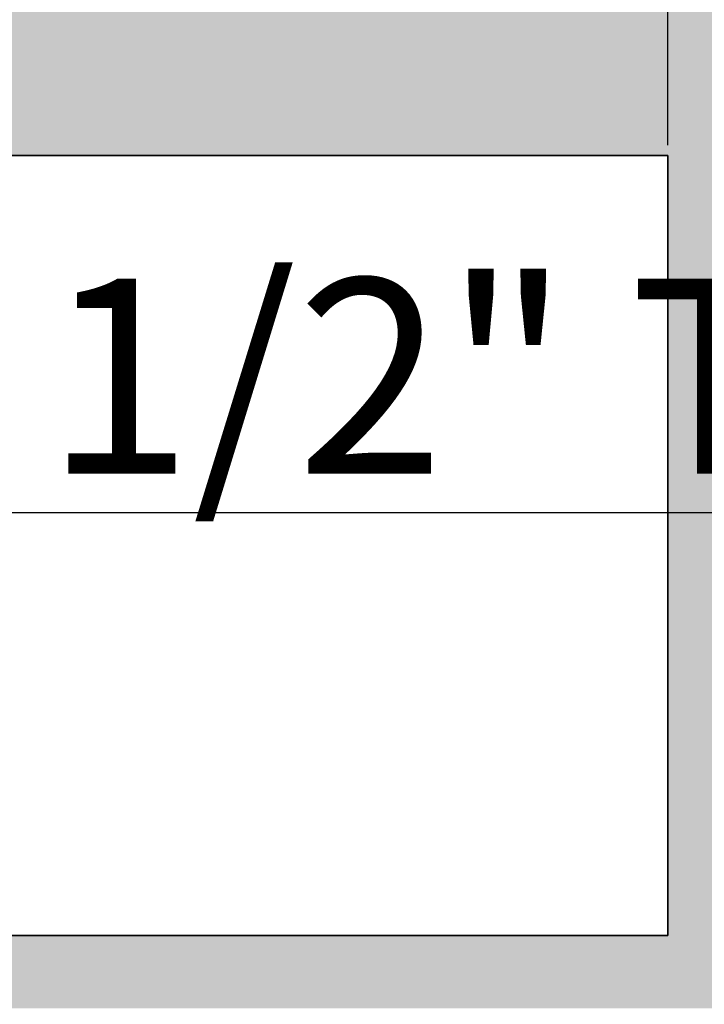
# Model space of a CAD drawing. Units: inches. Extents: x 2083 to 3317, y 1141 to 2115.
# Tile 20 of 256: x 2340 to 2382, y 1417 to 1477. Entities that reach past the tile are written whole.
import ezdxf

# ---------------------------------------------------------------- set-up
doc = ezdxf.new("R2010")
doc.units = ezdxf.units.IN
doc.layers.add('A-ANNO-DIMS', color=2, linetype='Continuous', lineweight=18)
doc.layers.add('A-WALL', color=7, linetype='Continuous', lineweight=35)
doc.layers.add('A-WALL-PATT', color=251, linetype='Continuous', lineweight=13, true_color=0x636466)
doc.styles.get("Standard").update_dxf_attribs({"font": 'arial.ttf'})
doc.dimstyles.new('ISO-25', dxfattribs={"dimtxt": 12, "dimasz": 12, "dimexe": 1.25, "dimexo": 0.625, "dimtad": 1, "dimlunit": 3, "dimtxsty": 'Standard', "dimcen": 2.5, "dimadec": 0, "dimazin": 0, "dimtfac": 1, "dimtmove": 0, "dimatfit": 3, "dimfxl": 1, "dimarcsym": 0})

# ---------------------------------------------------------------- blocks, each defined once
blk = doc.blocks.new('*D23')
at = {"layer": 'A-ANNO-DIMS', "color": 0, "lineweight": -2, "transparency": 16777216}
for p, q in [((2335.205, 1362.114), (2335.205, 1476.472)), ((2322.885, 1362.114), (2336.455, 1362.114)), ((2335.205, 1306.473), (2335.205, 1350.114)), ((2322.885, 1294.473), (2336.455, 1294.473))]:
    blk.add_line(p, q, dxfattribs=at)
at = {"layer": 'A-ANNO-DIMS', "color": 0, "transparency": 16777216}
for points in [[(2333.205, 1350.114), (2337.205, 1350.114), (2335.205, 1362.114)], [(2333.205, 1306.473), (2337.205, 1306.473), (2335.205, 1294.473)]]:
    blk.add_solid(points, dxfattribs=at)
at = {"layer": 'Defpoints', "color": 0, "transparency": 16777216}
for p in [(2322.26, 1362.114), (2335.205, 1362.114), (2322.26, 1294.473)]:
    blk.add_point(p, dxfattribs=at)
at = {"layer": 'A-ANNO-DIMS', "color": 0, "transparency": 16777216, "insert": (2328.376, 1425.293), "char_height": 12, "attachment_point": 5, "rotation": 90}
blk.add_mtext('5\'-7 1/2" TYP.', dxfattribs=at)
blk = doc.blocks.new('*D30')
at = {"layer": 'A-ANNO-DIMS', "color": 0, "lineweight": -2, "transparency": 16777216}
for p, q in [((2240.018, 1445.274), (2240.018, 1448.046)), ((2254.329, 1445.274), (2254.329, 1448.046)), ((2228.018, 1446.796), (2216.018, 1446.796)), ((2240.018, 1446.796), (2254.329, 1446.796)), ((2266.329, 1446.796), (2413.765, 1446.796))]:
    blk.add_line(p, q, dxfattribs=at)
at = {"layer": 'A-ANNO-DIMS', "color": 0, "transparency": 16777216}
for points in [[(2228.018, 1448.796), (2228.018, 1444.796), (2240.018, 1446.796)], [(2266.329, 1448.796), (2266.329, 1444.796), (2254.329, 1446.796)]]:
    blk.add_solid(points, dxfattribs=at)
at = {"layer": 'Defpoints', "color": 0, "transparency": 16777216}
for p in [(2254.329, 1446.796), (2240.018, 1444.649), (2254.329, 1444.649)]:
    blk.add_point(p, dxfattribs=at)
at = {"layer": 'A-ANNO-DIMS', "color": 0, "transparency": 16777216, "insert": (2346.047, 1453.625), "char_height": 12, "attachment_point": 5}
blk.add_mtext('WC 1\'-2 1/2" TYP.', dxfattribs=at)
blk = doc.blocks.new('*D62')
at = {"layer": 'A-ANNO-DIMS', "color": 0, "lineweight": -2, "transparency": 16777216}
for p, q in [((2235.96, 1469.386), (2235.96, 1522.361)), ((2379.96, 1469.386), (2379.96, 1522.361)), ((2247.96, 1521.111), (2367.96, 1521.111))]:
    blk.add_line(p, q, dxfattribs=at)
at = {"layer": 'A-ANNO-DIMS', "color": 0, "transparency": 16777216}
for points in [[(2247.96, 1523.111), (2247.96, 1519.111), (2235.96, 1521.111)], [(2367.96, 1523.111), (2367.96, 1519.111), (2379.96, 1521.111)]]:
    blk.add_solid(points, dxfattribs=at)
at = {"layer": 'Defpoints', "color": 0, "transparency": 16777216}
for p in [(2379.96, 1521.111), (2235.96, 1468.761), (2379.96, 1468.761)]:
    blk.add_point(p, dxfattribs=at)
at = {"layer": 'A-ANNO-DIMS', "color": 0, "transparency": 16777216, "insert": (2307.96, 1527.863), "char_height": 12, "attachment_point": 5}
blk.add_mtext('12\'-0"', dxfattribs=at)

msp = doc.modelspace()

# ---------------------------------------------------------------- hatches: boundary and pattern name
at = {"layer": 'A-WALL-PATT'}
h = msp.add_hatch(color=256, dxfattribs=at)
h.dxf.hatch_style = 1
h.paths.add_polyline_path([(3126.96, 2020.761), (2748.96, 2020.761), (2604.96, 2020.761), (2226.96, 2020.761), (2226.96, 1702.761), (2466.96, 1702.761), (2466.96, 1582.761), (2418.96, 1582.761), (2418.96, 1477.761), (2226.96, 1477.761), (2226.96, 1263.261), (2544.96, 1263.261), (2544.96, 1411.761), (2604.96, 1411.761), (2685.96, 1411.761), (2685.96, 1420.761), (2604.96, 1420.761), (2604.96, 1573.761), (2604.96, 1702.761), (2604.96, 2011.761), (2748.96, 2011.761), (2748.96, 1702.761), (2862.96, 1702.761), (2862.96, 1621.761), (2871.96, 1621.761), (2871.96, 1702.761), (2883.96, 1702.761), (2883.96, 1706.939, -0.026459), (2883.96, 1711.761), (2757.96, 1711.761), (2757.96, 1807.761), (2787.96, 1807.761), (2787.96, 1812.261), (2757.96, 1812.261), (2757.96, 2011.761), (2877.96, 2011.761), (2877.96, 1812.261), (2847.96, 1812.261), (2847.96, 1807.761), (2889.836, 1807.761), (2889.836, 1812.261), (2882.46, 1812.261), (2882.46, 2011.761), (3117.96, 2011.761), (3117.96, 1812.261), (2937.836, 1812.261), (2937.836, 1807.761), (2995.71, 1807.761), (2995.71, 1796.118), (3000.21, 1796.118), (3000.21, 1807.761), (3117.96, 1807.761), (3117.96, 1711.761), (3000.21, 1711.761), (3000.21, 1760.118), (2998.573, 1760.118, -0.020711), (2995.71, 1760.118), (2995.71, 1711.761), (2931.96, 1711.761), (2931.96, 1702.761), (3126.96, 1702.761)])
h.paths.add_polyline_path([(2471.46, 2011.761), (2471.46, 1810.011), (2462.717, 1810.011), (2462.717, 1805.511), (2505.96, 1805.511), (2505.96, 1810.011), (2475.96, 1810.011), (2475.96, 2011.761), (2595.96, 2011.761), (2595.96, 1810.011), (2565.96, 1810.011), (2565.96, 1805.511), (2595.96, 1805.511), (2595.96, 1711.761), (2235.96, 1711.761), (2235.96, 1805.511), (2353.71, 1805.511), (2353.71, 1796.054), (2358.21, 1796.054), (2358.21, 1805.511), (2414.717, 1805.511), (2414.717, 1810.011), (2235.96, 1810.011), (2235.96, 2011.761)], flags=16)
h.paths.add_polyline_path([(2270.205, 1994.61), (2270.205, 1970.61), (2246.205, 1970.61), (2246.205, 1994.61)], flags=0)
edge = h.paths.add_edge_path(flags=0)
edge.add_ellipse((2332.027, 1899.798), major_axis=(-3.043, 3.043), ratio=0.168252, start_angle=-161.33217, end_angle=-156.30711, ccw=False)
edge.add_ellipse((2333.082, 1898.744), major_axis=(-1.055, 1.055), ratio=0.453532, start_angle=-123.37102, end_angle=-94.15911)
edge = h.paths.add_edge_path(flags=0)
edge.add_ellipse((2332.027, 1968.876), major_axis=(3.043, 3.043), ratio=0.168252, start_angle=18.66783, end_angle=23.69289)
edge.add_spline(control_points=[(2332.926, 1970.691), (2332.227, 1970.336), (2330.894, 1969.659), (2328.413, 1970.932), (2327.204, 1967.749), (2324.71, 1969.956), (2322.533, 1967.012), (2320.013, 1971.296), (2317.68, 1968.158), (2316.041, 1967.102), (2315.427, 1966.81)], knot_values=[0, 0, 0, 0, 2.267059, 4.324559, 6.685584, 8.878641, 11.121502, 14.300359, 17.755284, 19.732645, 19.732645, 19.732645, 19.732645], degree=3, periodic=0)
edge.add_ellipse((2332.027, 1968.876), major_axis=(3.043, 3.043), ratio=0.168252, start_angle=18.66783, end_angle=23.69289, ccw=False)
edge.add_ellipse((2333.082, 1969.931), major_axis=(1.055, 1.055), ratio=0.453532, start_angle=56.62898, end_angle=85.84089, ccw=False)
edge = h.paths.add_edge_path(flags=0)
edge.add_spline(control_points=[(2296.428, 1967.988), (2293.628, 1965.336), (2287.704, 1959.727), (2299.744, 1949.996), (2294.533, 1935.669), (2290.573, 1920.604), (2293.394, 1909.974), (2296.185, 1904.967)], knot_values=[0.099185, 0.099185, 0.099185, 0.099185, 0.345301, 0.619822, 0.982653, 1.386093, 1.810555, 1.810555, 1.810555, 1.810555], degree=3, periodic=0)
edge.add_spline(control_points=[(2296.185, 1904.967), (2297.384, 1902.619), (2298.001, 1901.949), (2298.553, 1901.468)], knot_values=[0.006246, 0.006246, 0.006246, 0.006246, 0.055476, 0.055476, 0.055476, 0.055476], degree=3, periodic=0)
edge.add_spline(control_points=[(2298.553, 1901.468), (2297.259, 1900.923), (2295.225, 1900.232), (2293.06, 1900.614), (2292.101, 1900.788), (2292.09, 1900.791)], knot_values=[0.312835, 0.312835, 0.312835, 0.312835, 0.40178, 0.474987, 0.475903, 0.475903, 0.475903, 0.475903], degree=3, periodic=0)
edge.add_arc((2292.794, 1904.664), 3.937, 215.4209, 259.69818, ccw=False)
edge.add_spline(control_points=[(2289.585, 1902.382), (2289.477, 1902.535), (2289.368, 1902.688), (2289.261, 1902.841)], knot_values=[0.102872, 0.102872, 0.102872, 0.102872, 0.116896, 0.116896, 0.116896, 0.116896], degree=3, periodic=0)
edge.add_spline(control_points=[(2289.261, 1902.841), (2288.687, 1902.55), (2287.64, 1902.02), (2285.881, 1901.874), (2283.853, 1901.504), (2281.72, 1899.711), (2278.467, 1899.493), (2276.157, 1901.883), (2272.259, 1899.804), (2267.778, 1901.843), (2262.244, 1900.184), (2257.415, 1901.782), (2254.318, 1900.726), (2253.178, 1900.337)], knot_values=[0, 0, 0, 0, 1.907977, 3.477176, 5.261074, 7.972851, 11.680248, 13.717921, 16.939592, 22.789562, 27.502503, 33.595215, 37.145618, 37.145618, 37.145618, 37.145618], degree=3, periodic=0)
edge.add_line((2253.178, 1900.337), (2250.244, 1902.841))
edge.add_line((2250.244, 1902.841), (2250.244, 1965.833))
edge.add_line((2250.244, 1965.833), (2253.178, 1968.337))
edge.add_spline(control_points=[(2253.178, 1968.337), (2254.318, 1967.948), (2257.415, 1966.892), (2262.244, 1968.49), (2267.778, 1966.831), (2271.527, 1968.537), (2273.876, 1967.828), (2274.207, 1967.728)], knot_values=[0, 0, 0, 0, 0.09018, 0.244935, 0.364644, 0.513233, 0.537855, 0.537855, 0.537855, 0.537855], degree=3, periodic=0)
edge.add_arc((2274.353, 1963.793), 3.937, 72.05113, 92.12795, ccw=False)
edge.add_arc((2281.297, 1985.23), 18.596, 252.05113, 288.56572)
edge.add_arc((2292.317, 1956.029), 12.646, 71.02679, 113.77822, ccw=False)
edge = h.paths.add_edge_path(flags=0)
edge.add_spline(control_points=[(2274.899, 1951.856), (2275.066, 1951.617), (2275.233, 1951.377), (2275.398, 1951.136)], knot_values=[1.409916, 1.409916, 1.409916, 1.409916, 1.43159, 1.43159, 1.43159, 1.43159], degree=3, periodic=0)
edge.add_spline(control_points=[(2275.398, 1951.136), (2275.792, 1950.562), (2276.179, 1949.984), (2276.546, 1949.397)], knot_values=[1.358238, 1.358238, 1.358238, 1.358238, 1.409916, 1.409916, 1.409916, 1.409916], degree=3, periodic=0)
edge.add_line((2276.546, 1949.397), (2277.437, 1947.862))
edge.add_spline(control_points=[(2277.437, 1947.862), (2276.304, 1945.673), (2274.64, 1942.427), (2274.632, 1938.094), (2272.799, 1930.852), (2274.356, 1943.897), (2275.948, 1947.923), (2276.546, 1949.397)], knot_values=[0.005632, 0.005632, 0.005632, 0.005632, 0.186014, 0.266002, 0.357087, 0.59639, 0.739732, 0.739732, 0.739732, 0.739732], degree=3, periodic=0)
edge.add_spline(control_points=[(2276.546, 1949.397), (2276.179, 1949.984), (2275.792, 1950.562), (2275.398, 1951.136)], knot_values=[1.358238, 1.358238, 1.358238, 1.358238, 1.409916, 1.409916, 1.409916, 1.409916], degree=3, periodic=0)
edge.add_spline(control_points=[(2275.398, 1951.136), (2274.943, 1950.08), (2274.208, 1948.025), (2273.935, 1944.851), (2272.469, 1937.627), (2273.466, 1945.696), (2274.701, 1951.059), (2274.899, 1951.856)], knot_values=[0.104364, 0.104364, 0.104364, 0.104364, 0.189636, 0.269624, 0.36071, 0.600013, 0.644622, 0.644622, 0.644622, 0.644622], degree=3, periodic=0)
h.paths.add_polyline_path([(2269.168, 1963.128, -0.357527), (2268.171, 1960.976, -0.092561), (2268.171, 1939.436, -0.357527), (2269.168, 1937.285, -0.357527), (2267.016, 1938.282, -0.164785), (2254.686, 1938.282, -0.357527), (2252.534, 1937.285, -0.357527), (2253.531, 1939.436, -0.092561), (2253.531, 1960.976, -0.357527), (2252.534, 1963.128, -0.357527), (2254.686, 1962.131, -0.164785), (2267.016, 1962.131, -0.357527)], flags=0)
h.paths.add_polyline_path([(2248.874, 1967.802), (2248.874, 1957.028), (2249.458, 1957.028), (2249.458, 1911.647), (2248.874, 1911.647), (2248.874, 1900.873), (2246.512, 1900.873, 0.197327), (2244.15, 1902.457), (2244.15, 1966.218, 0.197327), (2246.512, 1967.802)], flags=0)
h.paths.add_polyline_path([(2269.168, 1931.389, -0.357527), (2268.171, 1929.238, -0.092561), (2268.171, 1907.698, -0.357527), (2269.168, 1905.547, -0.357527), (2267.016, 1906.544, -0.164785), (2254.686, 1906.544, -0.357527), (2252.534, 1905.547, -0.357527), (2253.531, 1907.698, -0.092561), (2253.531, 1929.238, -0.357527), (2252.534, 1931.389, -0.357527), (2254.686, 1930.392, -0.164785), (2267.016, 1930.392, -0.357527)], flags=0)
edge = h.paths.add_edge_path(flags=0)
edge.add_spline(control_points=[(2276.197, 1906.724), (2276.168, 1909.029), (2276.114, 1913.372), (2270.598, 1924.925), (2273.905, 1919.013), (2275.922, 1916.262), (2275.475, 1912.402), (2277.258, 1910.381), (2276.696, 1908.225), (2276.646, 1906.813), (2276.618, 1906.008)], knot_values=[0, 0, 0, 0, 8.61026, 16.221274, 18.843057, 23.804898, 27.440828, 29.356102, 31.203478, 33.650687, 33.650687, 33.650687, 33.650687], degree=3, periodic=0)
edge.add_spline(control_points=[(2276.618, 1906.008), (2276.623, 1905.624), (2276.498, 1904.629), (2275.442, 1903.855), (2274.937, 1903.08), (2274.859, 1902.841)], knot_values=[0.156488, 0.156488, 0.156488, 0.156488, 0.184398, 0.231376, 0.250598, 0.250598, 0.250598, 0.250598], degree=3, periodic=0)
edge.add_line((2274.859, 1902.841), (2276.506, 1902.841))
edge.add_spline(control_points=[(2276.506, 1902.841), (2276.788, 1903.085), (2277.665, 1904.125), (2278.25, 1904.341), (2277.654, 1908.527), (2278.156, 1906.228), (2278.1, 1905.286), (2278.847, 1904.069), (2277.857, 1903.415), (2277.874, 1902.991), (2277.904, 1902.841)], knot_values=[0.059574, 0.059574, 0.059574, 0.059574, 0.080753, 0.103741, 0.16972, 0.176036, 0.207137, 0.240474, 0.262341, 0.27366, 0.27366, 0.27366, 0.27366], degree=3, periodic=0)
edge.add_line((2277.904, 1902.841), (2280.03, 1902.841))
edge.add_spline(control_points=[(2280.03, 1902.841), (2279.888, 1903.088), (2279.499, 1903.982), (2280.152, 1905.939), (2278.104, 1909.658), (2279.762, 1907.185), (2280.328, 1904.875), (2280.485, 1903.49), (2281.463, 1903.249), (2281.758, 1902.936), (2281.834, 1902.841)], knot_values=[0.013856, 0.013856, 0.013856, 0.013856, 0.034874, 0.088867, 0.107879, 0.126738, 0.158714, 0.193757, 0.217487, 0.226722, 0.226722, 0.226722, 0.226722], degree=3, periodic=0)
edge.add_spline(control_points=[(2281.834, 1902.841), (2281.788, 1902.827), (2281.647, 1902.783), (2281.396, 1902.859), (2281.088, 1902.985), (2280.721, 1903.061), (2280.333, 1903.026), (2280.125, 1902.899), (2280.03, 1902.841)], knot_values=[0, 0, 0, 0, 0.14413, 0.435517, 0.749276, 1.153046, 1.548371, 1.878348, 1.878348, 1.878348, 1.878348], degree=3, periodic=0)
edge.add_line((2280.03, 1902.841), (2277.904, 1902.841))
edge.add_spline(control_points=[(2277.904, 1902.841), (2277.893, 1902.796), (2277.865, 1902.68), (2277.607, 1902.687), (2277.274, 1902.801), (2276.838, 1902.62), (2276.584, 1902.789), (2276.506, 1902.841)], knot_values=[0, 0, 0, 0, 0.127189, 0.326199, 0.628009, 1.24357, 1.515331, 1.515331, 1.515331, 1.515331], degree=3, periodic=0)
edge.add_line((2276.506, 1902.841), (2274.859, 1902.841))
edge.add_spline(control_points=[(2274.859, 1902.841), (2274.814, 1902.899), (2274.725, 1903.013), (2274.493, 1903.119), (2274.244, 1902.961), (2273.937, 1903.185), (2273.614, 1902.983), (2273.408, 1902.883), (2273.322, 1902.841)], knot_values=[0, 0, 0, 0, 0.21843, 0.436957, 0.687977, 0.990379, 1.398396, 1.69185, 1.69185, 1.69185, 1.69185], degree=3, periodic=0)
edge.add_spline(control_points=[(2273.322, 1902.841), (2273.617, 1903.446), (2274.274, 1904.538), (2276.027, 1904.574), (2276.207, 1906.584), (2276.197, 1906.724)], knot_values=[0.012227, 0.012227, 0.012227, 0.012227, 0.059472, 0.106218, 0.134458, 0.134458, 0.134458, 0.134458], degree=3, periodic=0)
h.paths.add_polyline_path([(2270.776, 1897.79), (2270.776, 1873.79), (2246.776, 1873.79), (2246.776, 1897.79)], flags=0)
h.paths.add_polyline_path([(2353.71, 1760.005), (2353.71, 1760.054), (2358.21, 1760.054, -0.033729)], flags=0)
h.paths.add_polyline_path([(2321.819, 1737.529), (2341.995, 1737.529, -0.414214), (2343.203, 1736.321), (2343.203, 1721.021, -0.414214), (2341.995, 1719.813), (2321.819, 1719.813, -0.414214), (2320.611, 1721.021), (2320.611, 1736.321, -0.414214)], flags=0)
h.paths.add_polyline_path([(2324.235, 1736.321), (2339.579, 1736.321, -0.414214), (2341.995, 1733.905), (2341.995, 1725.45, -0.414214), (2339.579, 1723.034), (2333.681, 1723.034), (2333.845, 1722.045, -0.870646), (2335.425, 1721.826, -0.767327), (2333.923, 1721.423), (2331.291, 1721.423, -0.767327), (2329.788, 1721.826, -0.870646), (2331.368, 1722.045), (2331.533, 1723.034), (2324.235, 1723.034, -0.414214), (2321.819, 1725.45), (2321.819, 1733.905, -0.414214)], flags=0)
h.paths.add_polyline_path([(2570.484, 1928.615), (2589.684, 1928.615), (2590.169, 1928.615), (2590.169, 1904.993), (2570.484, 1904.993)], flags=0)
h.paths.add_polyline_path([(2574.447, 1927.264, -1), (2572.829, 1927.264, -1)], flags=0)
h.paths.add_polyline_path([(2573.09, 1926.941), (2573.925, 1927.776), (2574.148, 1927.553), (2573.313, 1926.718)], flags=0)
h.paths.add_polyline_path([(2578.779, 1919.73, -1), (2571.592, 1919.73, -1)], flags=0)
h.paths.add_polyline_path([(2578.385, 1919.73, -1), (2571.985, 1919.73, -1)], flags=0)
h.paths.add_polyline_path([(2331.596, 1729.476, -1), (2333.618, 1729.476, -1)], flags=0)
h.paths.add_polyline_path([(2578.034, 1927.264, -1), (2576.416, 1927.264, -1)], flags=0)
h.paths.add_polyline_path([(2576.689, 1927.531), (2576.912, 1927.754), (2577.747, 1926.919), (2577.524, 1926.696)], flags=0)
h.paths.add_polyline_path([(2578.139, 1909.86, -1), (2572.232, 1909.86, -1)], flags=0)
h.paths.add_polyline_path([(2577.745, 1909.86, -1), (2572.625, 1909.86, -1)], flags=0)
h.paths.add_polyline_path([(2583.798, 1927.264, -1), (2582.179, 1927.264, -1)], flags=0)
h.paths.add_polyline_path([(2582.719, 1927.754), (2583.554, 1926.919), (2583.331, 1926.696), (2582.496, 1927.531)], flags=0)
h.paths.add_polyline_path([(2582.496, 1927.531), (2582.719, 1927.754), (2583.554, 1926.919), (2583.331, 1926.696)], flags=0)
h.paths.add_polyline_path([(2587.739, 1920.53, -1), (2581.832, 1920.53, -1)], flags=0)
h.paths.add_polyline_path([(2587.345, 1920.53, -1), (2582.225, 1920.53, -1)], flags=0)
h.paths.add_polyline_path([(2587.385, 1927.264, -1), (2585.766, 1927.264, -1)], flags=0)
h.paths.add_polyline_path([(2586.082, 1926.98), (2586.917, 1927.815), (2587.14, 1927.593), (2586.305, 1926.758)], flags=0)
h.paths.add_polyline_path([(2588.379, 1910.66, -1), (2581.192, 1910.66, -1)], flags=0)
h.paths.add_polyline_path([(2587.985, 1910.66, -1), (2581.585, 1910.66, -1)], flags=0)
h.paths.add_polyline_path([(2417.168, 1729.478), (2437.344, 1729.478, -0.414214), (2438.552, 1728.27), (2438.552, 1712.969, -0.414214), (2437.344, 1711.761), (2417.168, 1711.761, -0.414214), (2415.96, 1712.969), (2415.96, 1728.27, -0.414214)], flags=0)
h.paths.add_polyline_path([(2419.584, 1728.27), (2434.928, 1728.27, -0.414214), (2437.344, 1725.854), (2437.344, 1717.398, -0.414214), (2434.928, 1714.983), (2429.029, 1714.983), (2429.194, 1713.994, -0.870646), (2430.774, 1713.775, -0.767327), (2429.271, 1713.372), (2426.64, 1713.372, -0.767327), (2425.137, 1713.775, -0.870646), (2426.717, 1713.994), (2426.882, 1714.983), (2419.584, 1714.983, -0.414214), (2417.168, 1717.398), (2417.168, 1725.854, -0.414214)], flags=0)
h.paths.add_polyline_path([(2419.584, 1728.27), (2434.928, 1728.27, -0.414214), (2437.344, 1725.854), (2437.344, 1717.398, -0.414214), (2434.928, 1714.983), (2429.029, 1714.983), (2428.358, 1719.009), (2427.553, 1719.009), (2426.882, 1714.983), (2419.584, 1714.983, -0.414214), (2417.168, 1717.398), (2417.168, 1725.854, -0.414214)], flags=0)
h.paths.add_polyline_path([(2426.944, 1721.425, -1), (2428.967, 1721.425, -1)], flags=0)
h.paths.add_polyline_path([(2475.96, 1702.761), (2595.96, 1702.761), (2595.96, 1582.761), (2475.96, 1582.761)], flags=16)
h.paths.add_polyline_path([(2427.96, 1573.761), (2595.96, 1573.761), (2595.96, 1468.761), (2595.96, 1420.761), (2384.46, 1420.761), (2384.46, 1468.761), (2427.96, 1468.761)], flags=16)
h.paths.add_polyline_path([(2379.96, 1468.761), (2379.96, 1420.761), (2235.96, 1420.761), (2235.96, 1468.761)], flags=16)
h.paths.add_polyline_path([(2317.816, 1466.696), (2337.992, 1466.696, -0.414214), (2339.2, 1465.488), (2339.2, 1450.187, -0.414214), (2337.992, 1448.979), (2317.816, 1448.979, -0.414214), (2316.608, 1450.187), (2316.608, 1465.488, -0.414214)], flags=0)
h.paths.add_polyline_path([(2320.232, 1465.488), (2335.576, 1465.488, -0.414214), (2337.992, 1463.072), (2337.992, 1454.616, -0.414214), (2335.576, 1452.2), (2329.677, 1452.2), (2329.842, 1451.212, -0.870646), (2331.422, 1450.992, -0.767327), (2329.92, 1450.59), (2327.288, 1450.59, -0.767327), (2325.785, 1450.992, -0.870646), (2327.365, 1451.212), (2327.53, 1452.2), (2320.232, 1452.2, -0.414214), (2317.816, 1454.616), (2317.816, 1463.072, -0.414214)], flags=0)
h.paths.add_polyline_path([(2320.232, 1465.488), (2335.576, 1465.488, -0.414214), (2337.992, 1463.072), (2337.992, 1454.616, -0.414214), (2335.576, 1452.2), (2329.677, 1452.2), (2329.006, 1456.227), (2328.201, 1456.227), (2327.53, 1452.2), (2320.232, 1452.2, -0.414214), (2317.816, 1454.616), (2317.816, 1463.072, -0.414214)], flags=0)
h.paths.add_polyline_path([(2327.593, 1458.643, -1), (2329.615, 1458.643, -1)], flags=0)
h.paths.add_polyline_path([(2244.412, 1433.34), (2241.921, 1433.34, -0.414214), (2240.018, 1435.244), (2240.018, 1440.953, -0.414211), (2241.921, 1442.856), (2244.412, 1442.856, -1.976472)], flags=0)
h.paths.add_polyline_path([(2245.357, 1434.398, -0.414214), (2245.357, 1441.799, -2.144098)], flags=0)
h.paths.add_polyline_path([(2535.96, 1416.261), (2535.96, 1272.261), (2235.96, 1272.261), (2235.96, 1416.261)], flags=16)
h.paths.add_polyline_path([(2260.12, 1384.293), (2260.12, 1362.039), (2237.865, 1362.039), (2237.865, 1384.293)], flags=0)
edge = h.paths.add_edge_path(flags=0)
edge.add_line((2318.252, 1362.093), (2318.146, 1362.001))
edge.add_ellipse((2317.445, 1360.431), major_axis=(2.822, 2.822), ratio=0.168252, start_angle=18.66783, end_angle=20.94813, ccw=False)
edge.add_ellipse((2318.423, 1361.409), major_axis=(0.978, 0.978), ratio=0.453532, start_angle=56.62898, end_angle=70.2262, ccw=False)
edge = h.paths.add_edge_path(flags=0)
edge.add_line((2319.107, 1295.571), (2319.015, 1295.677))
edge.add_ellipse((2317.445, 1296.378), major_axis=(-2.822, 2.822), ratio=0.168252, start_angle=-161.33217, end_angle=-159.05187, ccw=False)
edge.add_ellipse((2318.423, 1295.4), major_axis=(-0.978, 0.978), ratio=0.453532, start_angle=-123.37102, end_angle=-109.7738)
edge = h.paths.add_edge_path(flags=0)
edge.add_spline(control_points=[(2284.21, 1301.17), (2284.581, 1300.445), (2284.891, 1299.892), (2285.16, 1299.461)], knot_values=[0.039066, 0.039066, 0.039066, 0.039066, 0.055476, 0.055476, 0.055476, 0.055476], degree=3, periodic=0)
edge.add_line((2285.16, 1299.461), (2284.21, 1301.17))
edge = h.paths.add_edge_path(flags=0)
edge.add_line((2280.412, 1297.298), (2283.37, 1297.036))
edge.add_line((2283.37, 1297.036), (2286.406, 1297.926))
edge.add_spline(control_points=[(2286.406, 1297.926), (2285.305, 1297.463), (2284.345, 1297.129), (2283.37, 1297.036)], knot_values=[0.394369, 0.394369, 0.394369, 0.394369, 0.475903, 0.475903, 0.475903, 0.475903], degree=3, periodic=0)
edge.add_spline(control_points=[(2283.37, 1297.036), (2283.281, 1297.028), (2282.316, 1296.957), (2281.313, 1297.134), (2280.423, 1297.296), (2280.412, 1297.298)], knot_values=[0.312835, 0.312835, 0.312835, 0.312835, 0.320246, 0.393453, 0.394369, 0.394369, 0.394369, 0.394369], degree=3, periodic=0)
edge = h.paths.add_edge_path(flags=0)
edge.add_line((2284.436, 1359.607), (2280.446, 1355.328))
edge.add_line((2280.446, 1355.328), (2279.58, 1351.018))
edge.add_line((2279.58, 1351.018), (2282.413, 1346.58))
edge.add_spline(control_points=[(2282.413, 1346.58), (2283.153, 1345.589), (2284.253, 1344.029), (2284.801, 1342.387), (2284.935, 1341.806)], knot_values=[1.240098, 1.240098, 1.240098, 1.240098, 1.332892, 1.382712, 1.382712, 1.382712, 1.382712], degree=3, periodic=0)
edge.add_spline(control_points=[(2284.935, 1341.806), (2285.319, 1340.141), (2285.233, 1338.409), (2284.91, 1336.654)], knot_values=[1.097484, 1.097484, 1.097484, 1.097484, 1.240098, 1.240098, 1.240098, 1.240098], degree=3, periodic=0)
edge.add_spline(control_points=[(2284.91, 1336.654), (2284.587, 1334.899), (2284.027, 1333.12), (2283.463, 1331.361)], knot_values=[0.95487, 0.95487, 0.95487, 0.95487, 1.097484, 1.097484, 1.097484, 1.097484], degree=3, periodic=0)
edge.add_line((2283.463, 1331.361), (2281.89, 1326.153))
edge.add_line((2281.89, 1326.153), (2280.756, 1321.056))
edge.add_line((2280.756, 1321.056), (2280.299, 1316.002))
edge.add_line((2280.299, 1316.002), (2280.716, 1310.95))
edge.add_line((2280.716, 1310.95), (2282.028, 1305.972))
edge.add_line((2282.028, 1305.972), (2284.21, 1301.17))
edge.add_spline(control_points=[(2284.21, 1301.17), (2283.341, 1302.73), (2282.612, 1304.336), (2282.028, 1305.972)], knot_values=[0.099185, 0.099185, 0.099185, 0.099185, 0.241799, 0.241799, 0.241799, 0.241799], degree=3, periodic=0)
edge.add_spline(control_points=[(2282.028, 1305.972), (2281.444, 1307.608), (2281.005, 1309.273), (2280.716, 1310.95)], knot_values=[0.241799, 0.241799, 0.241799, 0.241799, 0.384413, 0.384413, 0.384413, 0.384413], degree=3, periodic=0)
edge.add_spline(control_points=[(2280.716, 1310.95), (2280.433, 1312.588), (2280.289, 1314.277), (2280.299, 1315.962), (2280.299, 1316.002)], knot_values=[0.384413, 0.384413, 0.384413, 0.384413, 0.523647, 0.527028, 0.527028, 0.527028, 0.527028], degree=3, periodic=0)
edge.add_spline(control_points=[(2280.299, 1316.002), (2280.312, 1317.687), (2280.478, 1319.368), (2280.756, 1321.056)], knot_values=[0.527028, 0.527028, 0.527028, 0.527028, 0.669642, 0.669642, 0.669642, 0.669642], degree=3, periodic=0)
edge.add_spline(control_points=[(2280.756, 1321.056), (2281.035, 1322.744), (2281.426, 1324.44), (2281.89, 1326.153)], knot_values=[0.669642, 0.669642, 0.669642, 0.669642, 0.812256, 0.812256, 0.812256, 0.812256], degree=3, periodic=0)
edge.add_spline(control_points=[(2281.89, 1326.153), (2282.264, 1327.533), (2282.788, 1329.262), (2283.353, 1331.018), (2283.463, 1331.361)], knot_values=[0.812256, 0.812256, 0.812256, 0.812256, 0.927087, 0.95487, 0.95487, 0.95487, 0.95487], degree=3, periodic=0)
edge.add_line((2283.463, 1331.361), (2284.91, 1336.654))
edge.add_line((2284.91, 1336.654), (2284.935, 1341.806))
edge.add_line((2284.935, 1341.806), (2282.413, 1346.58))
edge.add_spline(control_points=[(2282.413, 1346.58), (2281.275, 1348.104), (2280.078, 1349.57), (2279.58, 1351.018)], knot_values=[1.382712, 1.382712, 1.382712, 1.382712, 1.525326, 1.525326, 1.525326, 1.525326], degree=3, periodic=0)
edge.add_spline(control_points=[(2279.58, 1351.018), (2279.443, 1351.415), (2279.136, 1352.857), (2279.735, 1354.29), (2280.446, 1355.328)], knot_values=[1.525326, 1.525326, 1.525326, 1.525326, 1.564439, 1.667941, 1.667941, 1.667941, 1.667941], degree=3, periodic=0)
edge.add_spline(control_points=[(2280.446, 1355.328), (2281.426, 1356.758), (2282.931, 1358.183), (2284.436, 1359.607)], knot_values=[1.667941, 1.667941, 1.667941, 1.667941, 1.810555, 1.810555, 1.810555, 1.810555], degree=3, periodic=0)
edge.add_arc((2280.623, 1348.518), 11.726, 71.02679, 113.77822)
edge.add_arc((2270.405, 1375.595), 17.244, 252.05113, 288.56572, ccw=False)
edge.add_arc((2263.966, 1355.718), 3.651, 72.05113, 92.12795)
edge.add_arc((2263.966, 1355.718), 3.651, 92.12795, 177.98513)
edge.add_spline(control_points=[(2260.318, 1355.846), (2260.26, 1354.221), (2260.551, 1350.187), (2262.999, 1346.766), (2264.473, 1344.649)], knot_values=[1.43159, 1.43159, 1.43159, 1.43159, 1.564144, 1.770695, 1.770695, 1.770695, 1.770695], degree=3, periodic=0)
edge.add_line((2264.473, 1344.649), (2264.936, 1343.983))
edge.add_spline(control_points=[(2263.801, 1340.248), (2263.843, 1340.514), (2264.067, 1341.756), (2264.513, 1343.002), (2264.935, 1343.981)], knot_values=[0.53657, 0.53657, 0.53657, 0.53657, 0.559349, 0.644622, 0.644622, 0.644622, 0.644622], degree=3, periodic=0)
edge.add_spline(control_points=[(2264.935, 1343.981), (2265.118, 1343.715), (2265.299, 1343.448), (2265.477, 1343.179)], knot_values=[1.384077, 1.384077, 1.384077, 1.384077, 1.409916, 1.409916, 1.409916, 1.409916], degree=3, periodic=0)
edge.add_spline(control_points=[(2265.477, 1343.179), (2265.655, 1342.911), (2265.829, 1342.641), (2265.999, 1342.369)], knot_values=[1.358238, 1.358238, 1.358238, 1.358238, 1.384077, 1.384077, 1.384077, 1.384077], degree=3, periodic=0)
edge.add_line((2265.999, 1342.369), (2266.826, 1340.946))
edge.add_spline(control_points=[(2266.826, 1340.946), (2268.894, 1337.09), (2271.398, 1325.843), (2270.516, 1310.569), (2275.919, 1301.861), (2277.79, 1299.199)], knot_values=[0.116896, 0.116896, 0.116896, 0.116896, 0.472987, 1.050969, 1.313793, 1.313793, 1.313793, 1.313793], degree=3, periodic=0)
edge.add_spline(control_points=[(2277.79, 1299.199), (2277.839, 1299.128), (2277.889, 1299.057), (2277.94, 1298.987)], knot_values=[0.109884, 0.109884, 0.109884, 0.109884, 0.116896, 0.116896, 0.116896, 0.116896], degree=3, periodic=0)
edge.add_line((2277.94, 1298.987), (2277.789, 1299.199))
edge.add_spline(control_points=[(2277.789, 1299.199), (2277.257, 1298.929), (2276.286, 1298.438), (2275.039, 1298.334), (2274.383, 1298.239), (2274.215, 1298.209)], knot_values=[33.12187, 33.12187, 33.12187, 33.12187, 35.029056, 36.598255, 37.144827, 37.144827, 37.144827, 37.144827], degree=3, periodic=0)
edge.add_line((2274.215, 1298.209), (2273.073, 1297.893))
edge.add_spline(control_points=[(2273.073, 1297.893), (2272.323, 1297.58), (2271.039, 1296.511), (2269.248, 1296.226), (2268.423, 1296.375)], knot_values=[26.532584, 26.532584, 26.532584, 26.532584, 29.198919, 31.839101, 31.839101, 31.839101, 31.839101], degree=3, periodic=0)
edge.add_line((2268.423, 1296.375), (2263.879, 1297.458))
edge.add_spline(control_points=[(2263.879, 1297.458), (2263.556, 1297.359), (2261.86, 1296.839), (2260.239, 1297.282), (2258.933, 1297.516)], knot_values=[15.919551, 15.919551, 15.919551, 15.919551, 16.939592, 21.226067, 21.226067, 21.226067, 21.226067], degree=3, periodic=0)
edge.add_line((2258.933, 1297.516), (2254.055, 1297.329))
edge.add_spline(control_points=[(2254.055, 1297.329), (2253.756, 1297.296), (2252.114, 1297.165), (2250.462, 1297.544), (2249.13, 1297.668)], knot_values=[5.306517, 5.306517, 5.306517, 5.306517, 6.276435, 10.613034, 10.613034, 10.613034, 10.613034], degree=3, periodic=0)
edge.add_line((2249.13, 1297.668), (2244.332, 1296.878))
edge.add_line((2244.332, 1296.878), (2241.611, 1299.199))
edge.add_line((2241.611, 1299.199), (2241.611, 1357.609))
edge.add_line((2241.611, 1357.609), (2244.332, 1359.931))
edge.add_line((2244.332, 1359.931), (2252.729, 1359.543))
edge.add_spline(control_points=[(2252.729, 1359.543), (2252.871, 1359.546), (2253.306, 1359.548), (2253.74, 1359.514), (2254.032, 1359.482)], knot_values=[0.233291, 0.233291, 0.233291, 0.233291, 0.244935, 0.268927, 0.268927, 0.268927, 0.268927], degree=3, periodic=0)
edge.add_line((2254.032, 1359.482), (2259.587, 1359.416))
edge.add_spline(control_points=[(2259.587, 1359.416), (2260.677, 1359.629), (2262.073, 1359.897), (2263.524, 1359.459), (2263.83, 1359.366)], knot_values=[0.422516, 0.422516, 0.422516, 0.422516, 0.513233, 0.537855, 0.537855, 0.537855, 0.537855], degree=3, periodic=0)
edge.add_arc((2263.966, 1355.718), 3.651, 72.05113, 92.12795, ccw=False)
edge.add_arc((2270.405, 1375.595), 17.244, 252.05113, 288.56572)
edge.add_arc((2280.623, 1348.518), 11.726, 71.02679, 113.77822, ccw=False)
h.paths.add_polyline_path([(2240.341, 1359.435), (2240.341, 1349.444), (2240.882, 1349.444), (2240.882, 1307.365), (2240.341, 1307.365), (2240.341, 1297.374), (2238.15, 1297.374, 0.197327), (2235.96, 1298.843), (2235.96, 1357.966, 0.197327), (2238.15, 1359.435)], flags=0)
h.paths.add_polyline_path([(2259.158, 1355.101, -0.357527), (2258.233, 1353.106, -0.092561), (2258.233, 1333.133, -0.357527), (2259.158, 1331.138, -0.357527), (2257.163, 1332.062, -0.164785), (2245.729, 1332.062, -0.357527), (2243.735, 1331.138, -0.357527), (2244.659, 1333.133, -0.092561), (2244.659, 1353.106, -0.357527), (2243.735, 1355.101, -0.357527), (2245.729, 1354.176, -0.164785), (2257.163, 1354.176, -0.357527)], flags=0)
edge = h.paths.add_edge_path(flags=0)
edge.add_line((2265.999, 1342.369), (2266.826, 1340.946))
edge.add_line((2266.826, 1340.946), (2265.308, 1337.814))
edge.add_line((2265.308, 1337.814), (2264.358, 1334.653))
edge.add_line((2264.358, 1334.653), (2264.262, 1333.8))
edge.add_spline(control_points=[(2264.262, 1333.8), (2264.208, 1333.187), (2264.162, 1332.366), (2264.007, 1331.414), (2263.969, 1331.202)], knot_values=[0.464444, 0.464444, 0.464444, 0.464444, 0.516691, 0.531608, 0.531608, 0.531608, 0.531608], degree=3, periodic=0)
edge.add_spline(control_points=[(2263.969, 1331.202), (2263.775, 1330.119), (2263.424, 1328.791), (2263.257, 1328.531), (2263.234, 1328.515)], knot_values=[0.372682, 0.372682, 0.372682, 0.372682, 0.44885, 0.464444, 0.464444, 0.464444, 0.464444], degree=3, periodic=0)
edge.add_spline(control_points=[(2263.234, 1328.515), (2263.096, 1328.42), (2263.131, 1329.301), (2263.275, 1330.616)], knot_values=[0.280919, 0.280919, 0.280919, 0.280919, 0.372682, 0.372682, 0.372682, 0.372682], degree=3, periodic=0)
edge.add_spline(control_points=[(2263.275, 1330.616), (2263.419, 1331.93), (2263.672, 1333.677), (2263.97, 1335.315)], knot_values=[0.189157, 0.189157, 0.189157, 0.189157, 0.280919, 0.280919, 0.280919, 0.280919], degree=3, periodic=0)
edge.add_spline(control_points=[(2263.97, 1335.315), (2264.1, 1336.032), (2264.419, 1337.622), (2264.755, 1338.864), (2264.947, 1339.491)], knot_values=[0.097394, 0.097394, 0.097394, 0.097394, 0.137578, 0.189157, 0.189157, 0.189157, 0.189157], degree=3, periodic=0)
edge.add_spline(control_points=[(2264.947, 1339.491), (2265.29, 1340.606), (2265.644, 1341.494), (2265.999, 1342.369)], knot_values=[0.005632, 0.005632, 0.005632, 0.005632, 0.097394, 0.097394, 0.097394, 0.097394], degree=3, periodic=0)
h.paths.add_polyline_path([(2259.158, 1325.671, -0.357527), (2258.233, 1323.676, -0.092561), (2258.233, 1303.703, -0.357527), (2259.158, 1301.708, -0.357527), (2257.163, 1302.633, -0.164785), (2245.729, 1302.633, -0.357527), (2243.735, 1301.708, -0.357527), (2244.659, 1303.703, -0.092561), (2244.659, 1323.676, -0.357527), (2243.735, 1325.671, -0.357527), (2245.729, 1324.747, -0.164785), (2257.163, 1324.747, -0.357527)], flags=0)
edge = h.paths.add_edge_path(flags=0)
edge.add_spline(control_points=[(2261.709, 1317.311), (2261.679, 1317.418), (2261.762, 1317.389), (2262.491, 1316.09), (2262.962, 1315.301)], knot_values=[14.955861, 14.955861, 14.955861, 14.955861, 16.221274, 18.694826, 18.694826, 18.694826, 18.694826], degree=3, periodic=0)
edge.add_spline(control_points=[(2262.962, 1315.301), (2262.99, 1315.254), (2263.702, 1314.067), (2264.349, 1313.127), (2264.73, 1312.164)], knot_values=[18.694826, 18.694826, 18.694826, 18.694826, 18.843057, 22.433791, 22.433791, 22.433791, 22.433791], degree=3, periodic=0)
edge.add_spline(control_points=[(2264.73, 1312.164), (2264.876, 1311.796), (2265.177, 1310.77), (2265.143, 1309.559), (2265.248, 1308.824)], knot_values=[22.433791, 22.433791, 22.433791, 22.433791, 23.804898, 26.172756, 26.172756, 26.172756, 26.172756], degree=3, periodic=0)
edge.add_line((2265.248, 1308.824), (2265.851, 1307.172))
edge.add_spline(control_points=[(2265.851, 1307.172), (2266.065, 1306.822), (2266.384, 1306.332), (2266.424, 1305.781), (2266.42, 1305.611)], knot_values=[28.062562, 28.062562, 28.062562, 28.062562, 29.356102, 29.911721, 29.911721, 29.911721, 29.911721], degree=3, periodic=0)
edge.add_spline(control_points=[(2266.42, 1305.611), (2266.416, 1305.433), (2266.394, 1305.25), (2266.365, 1305.066)], knot_values=[29.911721, 29.911721, 29.911721, 29.911721, 30.497837, 30.497837, 30.497837, 30.497837], degree=3, periodic=0)
edge.add_line((2266.365, 1305.066), (2266.066, 1302.136))
edge.add_spline(control_points=[(2266.066, 1302.136), (2266.071, 1301.78), (2265.998, 1301.2), (2265.663, 1300.759), (2265.509, 1300.586)], knot_values=[0.156488, 0.156488, 0.156488, 0.156488, 0.184398, 0.203543, 0.203543, 0.203543, 0.203543], degree=3, periodic=0)
edge.add_line((2265.509, 1300.586), (2264.435, 1299.199))
edge.add_line((2264.435, 1299.199), (2265.962, 1299.199))
edge.add_line((2265.962, 1299.199), (2267.336, 1301.175))
edge.add_line((2267.336, 1301.175), (2267.312, 1301.986))
edge.add_spline(control_points=[(2267.312, 1301.986), (2267.261, 1302.862), (2267.16, 1303.737), (2267.271, 1303.326)], knot_values=[0.126229, 0.126229, 0.126229, 0.126229, 0.166617, 0.166617, 0.166617, 0.166617], degree=3, periodic=0)
edge.add_spline(control_points=[(2267.271, 1303.326), (2267.28, 1303.294), (2267.31, 1303.175), (2267.373, 1302.884), (2267.406, 1302.683), (2267.418, 1302.601)], knot_values=[0.166617, 0.166617, 0.166617, 0.166617, 0.16972, 0.176036, 0.180765, 0.180765, 0.180765, 0.180765], degree=3, periodic=0)
edge.add_spline(control_points=[(2267.744, 1300.988), (2267.688, 1301.151), (2267.481, 1301.657), (2267.484, 1302.145), (2267.418, 1302.601)], knot_values=[0.180765, 0.180765, 0.180765, 0.180765, 0.193767, 0.220139, 0.220139, 0.220139, 0.220139], degree=3, periodic=0)
edge.add_line((2267.418, 1302.601), (2267.744, 1300.988))
edge.add_spline(control_points=[(2267.744, 1300.988), (2267.832, 1300.732), (2267.932, 1300.31), (2267.555, 1299.975), (2267.429, 1299.829)], knot_values=[0.220139, 0.220139, 0.220139, 0.220139, 0.240474, 0.25489, 0.25489, 0.25489, 0.25489], degree=3, periodic=0)
edge.add_line((2267.429, 1299.829), (2267.258, 1299.199))
edge.add_line((2267.258, 1299.199), (2269.23, 1299.199))
edge.add_spline(control_points=[(2269.23, 1299.199), (2269.099, 1299.429), (2268.843, 1300.016), (2269.012, 1300.916), (2268.947, 1301.661)], knot_values=[0.013856, 0.013856, 0.013856, 0.013856, 0.034874, 0.067073, 0.067073, 0.067073, 0.067073], degree=3, periodic=0)
edge.add_line((2268.947, 1301.661), (2268.432, 1303.603))
edge.add_spline(control_points=[(2268.432, 1303.603), (2268.176, 1304.192), (2267.596, 1305.251), (2268.041, 1304.623), (2268.251, 1304.282)], knot_values=[0.090155, 0.090155, 0.090155, 0.090155, 0.107879, 0.120289, 0.120289, 0.120289, 0.120289], degree=3, periodic=0)
edge.add_spline(control_points=[(2268.251, 1304.282), (2268.361, 1304.105), (2269.058, 1302.918), (2269.383, 1301.59), (2269.521, 1300.776), (2269.575, 1300.556)], knot_values=[0.120289, 0.120289, 0.120289, 0.120289, 0.126738, 0.158714, 0.173506, 0.173506, 0.173506, 0.173506], degree=3, periodic=0)
edge.add_line((2269.575, 1300.556), (2270.686, 1299.421))
edge.add_spline(control_points=[(2270.686, 1299.421), (2270.767, 1299.357), (2270.838, 1299.281), (2270.903, 1299.199)], knot_values=[0.21816, 0.21816, 0.21816, 0.21816, 0.226722, 0.226722, 0.226722, 0.226722], degree=3, periodic=0)
edge.add_line((2270.937, 1299.193), (2270.903, 1299.199))
edge.add_spline(control_points=[(2270.903, 1299.199), (2270.86, 1299.186), (2270.73, 1299.146), (2270.496, 1299.216), (2270.272, 1299.308), (2270.121, 1299.348), (2270.063, 1299.36)], knot_values=[0.939174, 0.939174, 0.939174, 0.939174, 1.083304, 1.374691, 1.68845, 1.878348, 1.878348, 1.878348, 1.878348], degree=3, periodic=0)
edge.add_line((2270.063, 1299.36), (2269.23, 1299.199))
edge.add_line((2269.23, 1299.199), (2267.258, 1299.199))
edge.add_spline(control_points=[(2267.258, 1299.199), (2267.248, 1299.157), (2267.223, 1299.05), (2266.984, 1299.057), (2266.809, 1299.116), (2266.677, 1299.109), (2266.637, 1299.105)], knot_values=[0.757665, 0.757665, 0.757665, 0.757665, 0.884854, 1.083864, 1.385675, 1.515331, 1.515331, 1.515331, 1.515331], degree=3, periodic=0)
edge.add_spline(control_points=[(2266.637, 1299.105), (2266.485, 1299.089), (2266.236, 1299.017), (2266.035, 1299.151), (2265.962, 1299.199)], knot_values=[0, 0, 0, 0, 0.485905, 0.757665, 0.757665, 0.757665, 0.757665], degree=3, periodic=0)
edge.add_line((2265.962, 1299.199), (2264.435, 1299.199))
edge.add_line((2264.435, 1299.199), (2263.858, 1299.367))
edge.add_spline(control_points=[(2263.858, 1299.367), (2263.819, 1299.371), (2263.78, 1299.386), (2263.74, 1299.402)], knot_values=[0.845925, 0.845925, 0.845925, 0.845925, 0.978627, 0.978627, 0.978627, 0.978627], degree=3, periodic=0)
edge.add_line((2263.722, 1299.396), (2263.01, 1299.199))
edge.add_spline(control_points=[(2263.01, 1299.199), (2263.246, 1299.683), (2263.506, 1300.128), (2263.873, 1300.408)], knot_values=[0.012227, 0.012227, 0.012227, 0.012227, 0.052971, 0.052971, 0.052971, 0.052971], degree=3, periodic=0)
edge.add_spline(control_points=[(2263.873, 1300.408), (2263.932, 1300.453), (2264.084, 1300.553), (2264.255, 1300.624), (2264.36, 1300.665)], knot_values=[0.052971, 0.052971, 0.052971, 0.052971, 0.059472, 0.069086, 0.069086, 0.069086, 0.069086], degree=3, periodic=0)
edge.add_line((2264.36, 1300.665), (2265.142, 1301.078))
edge.add_line((2265.142, 1301.078), (2265.676, 1302.8))
edge.add_line((2265.676, 1302.8), (2265.541, 1305.704))
edge.add_line((2265.541, 1305.704), (2264.803, 1309.328))
edge.add_line((2264.803, 1309.328), (2263.041, 1314.092))
edge.add_spline(control_points=[(2263.041, 1314.092), (2262.384, 1315.671), (2261.796, 1316.998), (2261.709, 1317.311)], knot_values=[11.216896, 11.216896, 11.216896, 11.216896, 14.955861, 14.955861, 14.955861, 14.955861], degree=3, periodic=0)
h.paths.add_polyline_path([(2871.96, 1416.261), (2895.91, 1416.261), (2895.91, 1420.761), (2871.96, 1420.761), (2871.96, 1501.761), (2862.96, 1501.761), (2862.96, 1420.761), (2805.96, 1420.761), (2805.96, 1411.761), (2862.96, 1411.761), (2862.96, 1263.261), (3126.96, 1263.261), (3126.96, 1411.761), (3126.96, 1486.761), (2943.96, 1486.761), (2943.96, 1477.761), (2967.86, 1477.761), (2967.86, 1420.761), (2943.91, 1420.761), (2943.91, 1416.261), (3117.96, 1416.261), (3117.96, 1420.761), (2972.36, 1420.761), (2972.36, 1477.761), (3117.96, 1477.761), (3117.96, 1420.761), (3117.96, 1272.261), (2871.96, 1272.261)], flags=0)
h.paths.add_polyline_path([(2457.126, 1485.943), (2527.603, 1485.943), (2527.603, 1537.636), (2457.126, 1537.636)], flags=8)
h.paths.add_polyline_path([(2481.005, 1609.982), (2590.766, 1609.982), (2590.766, 1682.003), (2481.005, 1682.003)], flags=8)
h.paths.add_polyline_path([(2483.085, 1729.127), (2553.562, 1729.127), (2553.562, 1780.82), (2483.085, 1780.82)], flags=8)

# ---------------------------------------------------------------- linework, layer by layer
at = {"layer": 'A-WALL'}
for p, q in [((2235.96, 1468.761), (2379.96, 1468.761)), ((2235.96, 1468.761), (2379.96, 1468.761)), ((2379.96, 1468.761), (2379.96, 1420.761)), ((2379.96, 1468.761), (2379.96, 1420.761)), ((2235.96, 1420.761), (2379.96, 1420.761)), ((2379.96, 1420.761), (2235.96, 1420.761))]:
    msp.add_line(p, q, dxfattribs=at)

# ---------------------------------------------------------------- dimensions: what is measured, and where the dimension line sits
at = {"layer": 'A-ANNO-DIMS'}
dim = msp.add_linear_dim(base=(2379.96, 1521.111), p1=(2235.96, 1468.761), p2=(2379.96, 1468.761), dimstyle='ISO-25', override={"dimdec": 1, "dimlfac": 1, "dimrnd": 0, "dimzin": 1, "dimdsep": 46, "dimlunit": 4, "dimfrac": 2}, dxfattribs=at)
dim.commit()
dim.dimension.update_dxf_attribs({"geometry": '*D62', "text_midpoint": (2307.96, 1527.863)})
dim = msp.add_linear_dim(base=(2254.329, 1446.796), p1=(2240.018, 1444.649), p2=(2254.329, 1444.649), text='WC <> TYP.', dimstyle='ISO-25', override={"dimdec": 1, "dimlfac": 1, "dimrnd": 0, "dimzin": 1, "dimdsep": 46, "dimlunit": 4, "dimfrac": 2}, dxfattribs=at)
dim.commit()
dim.dimension.update_dxf_attribs({"geometry": '*D30', "text_midpoint": (2346.047, 1453.625)})
dim = msp.add_linear_dim(base=(2335.205, 1362.114), p1=(2322.26, 1294.473), p2=(2322.26, 1362.114), angle=90, text='<> TYP.', dimstyle='ISO-25', override={"dimdec": 1, "dimlfac": 1, "dimrnd": 0, "dimzin": 1, "dimdsep": 46, "dimlunit": 4, "dimfrac": 2}, dxfattribs=at)
dim.commit()
dim.dimension.update_dxf_attribs({"geometry": '*D23', "text_midpoint": (2328.376, 1425.293)})

doc.saveas('drawing.dxf')
